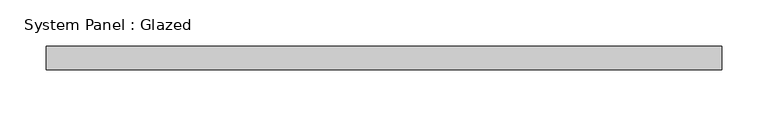
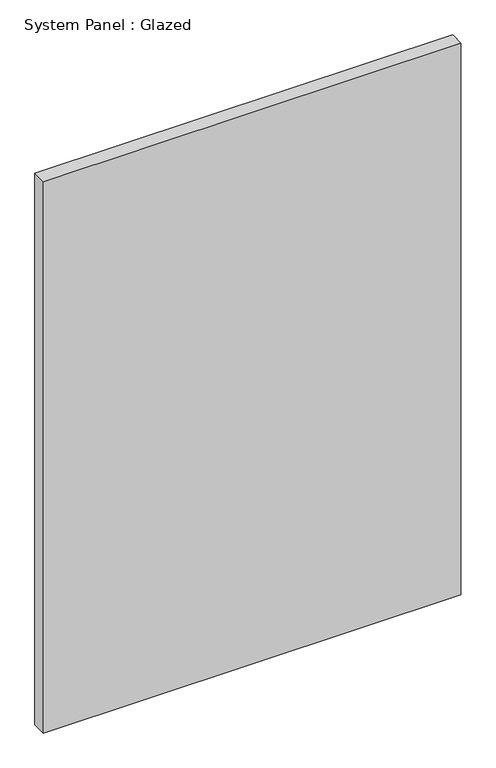
"""IFC4 building model written with IfcOpenShell, lengths in millimetres: plate geometry, System Panel : Glazed."""

from ifc_helpers import new_model, si_unit, origin, origin_with_axes, place, context, project, spatial, polyline, outline, extrude, source, transform, mapped, element, save


def system_panel_glazed_993ccbbe(model_context):
    return source(origin(), model_context, "Body", "SweptSolid", [
        extrude(outline(polyline([(366.1833333, 19.05), (-366.1833333, 19.05), (-366.1833333, 44.45), (366.1833333, 44.45), (366.1833333, 19.05)])), origin_with_axes(), (0.0, 0.0, 1.0), 1022.35),
    ])


if __name__ == "__main__":
    model = new_model("IFC4")
    model_context = context("Model", 3, world=origin())
    ifc_project = project(units=[si_unit("LENGTHUNIT", "METRE", prefix="MILLI")], contexts=[model_context])
    site = spatial("IfcSite", under=ifc_project)
    building = spatial("IfcBuilding", under=site)
    placement = place(None, origin())
    system_panel_glazed_shape = system_panel_glazed_993ccbbe(model_context)
    element("IfcPlate", 1, ObjectType="System Panel : Glazed", at=placement, inside=building, context=model_context, shape_type="MappedRepresentation", body=[
        mapped(system_panel_glazed_shape, transform((0.0, 0.0, 0.0), x_axis=(1.0, 0.0, 0.0), y_axis=(0.0, 1.0, 0.0), z_axis=(0.0, 0.0, 1.0))),
    ])
    save(model, "model.ifc")

# Revit data of these elements
# Type "System Panel : Glazed"
#   Construction Type Id = "GSP4R"
#   Analytic Construction = "1/8 in Pilkington single glazing"
#   Visual Light Transmittance = 0.9
#   Solar Heat Gain Coefficient = 0.86
#   Heat Transfer Coefficient (U) = 1.18115 BTU/(h·ft²·°F)
# Element 1 (IfcPlate, "System Panel : Glazed")
#   Materials on its faces: "Glass"
# Materials
#   "Glass": class "Glass", colour RGB 0 128 192, transparency 0.75, Description = "Soda Lime Glass", Cost = 0
